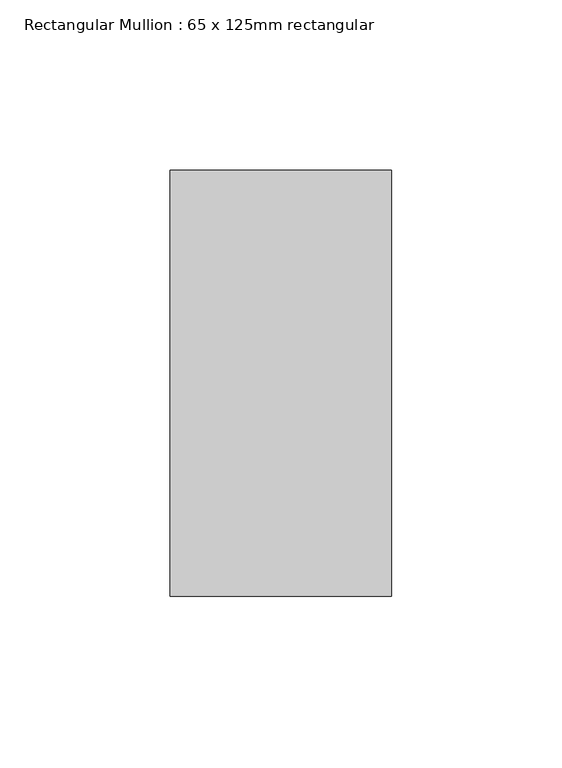
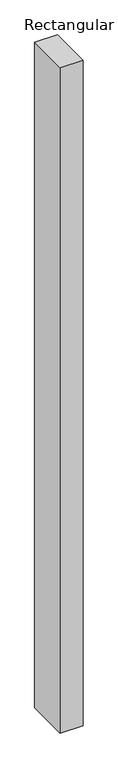
"""IFC4 building model written with IfcOpenShell, lengths in millimetres: member geometry, Rectangular Mullion : 65 x 125mm rectangular."""

from ifc_helpers import new_model, si_unit, frame, origin, place, context, project, spatial, polyline, outline, extrude, source, transform, mapped, element, save


def rectangular_mullion_65_x_125mm_rectangular_d57ab73f(model_context):
    return source(origin(), model_context, "Body", "SweptSolid", [
        extrude(outline(polyline([(0.0, 62.5), (0.0, -62.5), (-65.0, -62.5), (-65.0, 62.5), (0.0, 62.5)])), frame((0.0, 0.0, -2000.0), z_axis=(0.0, 0.0, 1.0), x_axis=(1.0, 0.0, 0.0)), (0.0, 0.0, 1.0), 2000.0),
    ])


if __name__ == "__main__":
    model = new_model("IFC4")
    model_context = context("Model", 3, world=origin())
    ifc_project = project(units=[si_unit("LENGTHUNIT", "METRE", prefix="MILLI")], contexts=[model_context])
    site = spatial("IfcSite", under=ifc_project)
    building = spatial("IfcBuilding", under=site)
    placement = place(None, origin())
    rectangular_mullion_65_x_125mm_rectangular_shape = rectangular_mullion_65_x_125mm_rectangular_d57ab73f(model_context)
    element("IfcMember", 1, ObjectType="Rectangular Mullion : 65 x 125mm rectangular", at=placement, inside=building, context=model_context, shape_type="MappedRepresentation", body=[
        mapped(rectangular_mullion_65_x_125mm_rectangular_shape, transform((0.0, 0.0, 0.0), x_axis=(1.0, 0.0, 0.0), y_axis=(0.0, 1.0, 0.0), z_axis=(0.0, 0.0, 1.0))),
    ])
    save(model, "model.ifc")

# Revit data of these elements
# Type "Rectangular Mullion : 65 x 125mm rectangular"
#   built-in parameter 1007304 = 0.410105 (stored number, unit not read)
#   built-in parameter 1007301 = 0.106627 (stored number, unit not read)
#   built-in parameter 1007300 = 0.106627 (stored number, unit not read)
# Element 1 (IfcMember, "Rectangular Mullion : 65 x 125mm rectangular")
#   Materials on its faces: "Aluminum"
# Materials
#   "Aluminum": class "Metal", colour RGB 244 245 246, transparency 0, Description = "Aluminum 6061", Cost = 0
